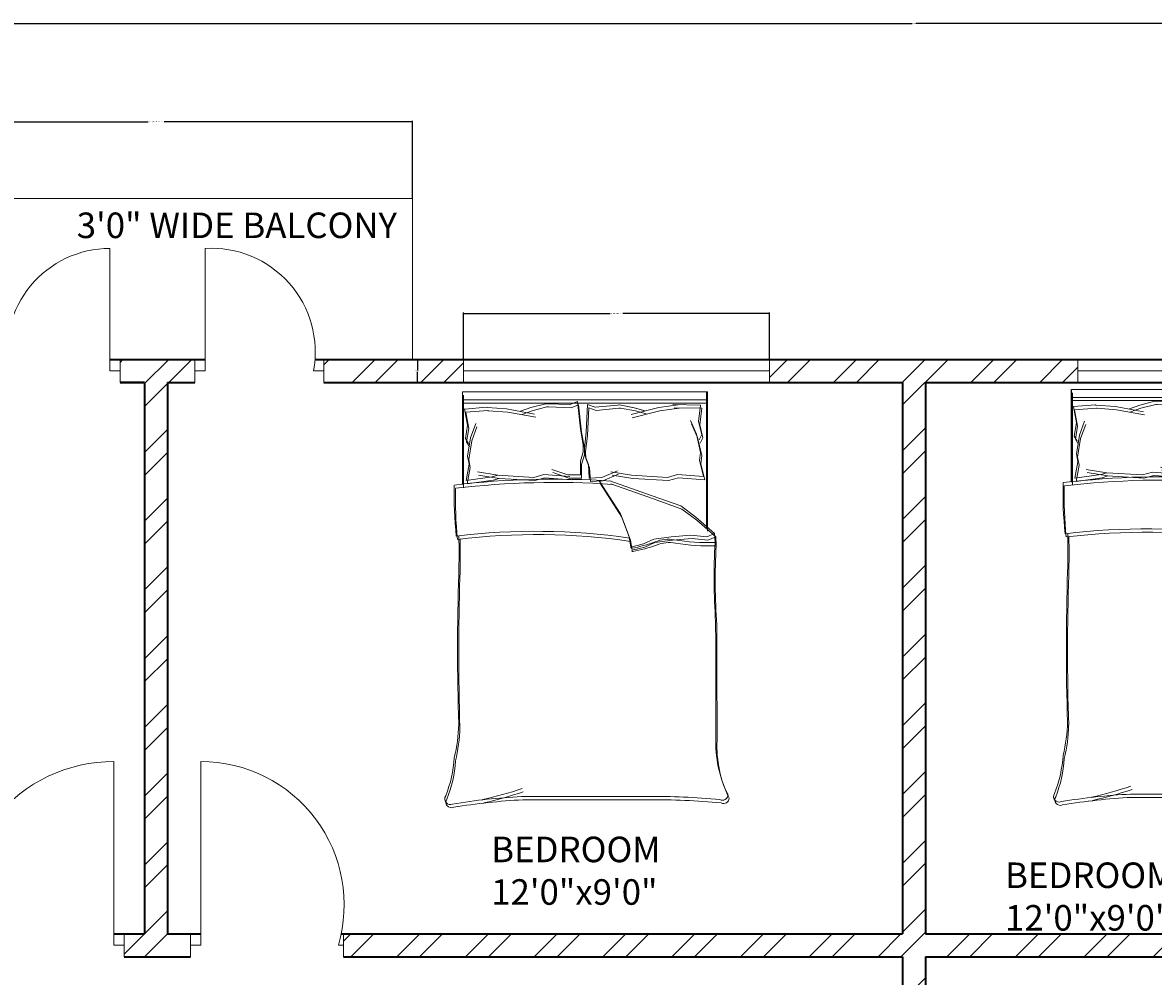
# Model space of a CAD drawing. Units: inches. Extents: x 2165 to 3042, y 1626 to 2968.
# Tile 5 of 11: x 2411 to 2633, y 2211 to 2398. Entities that reach past the tile are written whole.
import ezdxf

# ---------------------------------------------------------------- set-up
doc = ezdxf.new("R2010")
doc.units = ezdxf.units.IN
for name, color, linetype, lineweight in [('A-ANNO-DIMS', 2, 'Continuous', 18), ('A-AREA-IDEN', 7, 'Continuous', 18), ('A-DOOR', 3, 'Continuous', 18), ('A-FLOR-BALC', 7, 'Continuous', 18), ('A-FURN', 8, 'Continuous', 13), ('A-GLAZ', 4, 'Continuous', 18), ('A-WALL', 7, 'Continuous', 35), ('A-WALL-PATT', 252, 'Continuous', 13)]:
    doc.layers.add(name, color=color, linetype=linetype, lineweight=lineweight)
doc.styles.get("Standard").update_dxf_attribs({"font": 'arial.ttf'})
doc.dimstyles.get("Standard").update_dxf_attribs({"dimtxt": 0.18, "dimasz": 0.18, "dimexe": 0.18, "dimexo": 0.0625, "dimgap": 0.09, "dimtad": 0, "dimtih": 1, "dimtoh": 1, "dimdec": 4, "dimzin": 0, "dimdsep": 46, "dimtxsty": 'Standard', "dimcen": 0.09, "dimadec": 0, "dimazin": 0, "dimtfac": 1, "dimtdec": 4, "dimtofl": 0, "dimtmove": 0, "dimatfit": 3, "dimfxl": 1, "dimtolj": 1, "dimtzin": 0, "dimarcsym": 0})

# ---------------------------------------------------------------- blocks, each defined once
blk = doc.blocks.new('BED-DOUBLE')
for p, q in [((30.13, 53.18), (28.39, 53.1, 3.87)), ((30.13, 53.18), (28.39, 53.1, 3.87)), ((0, 51.27), (0, 51.49)), ((0, 51.49), (0.64, 51.49)), ((0, 51.27), (26.61, 51.27)), ((0, 51.27), (26.61, 51.27)), ((0, 51.27), (0, 3.48)), ((0.64, 51.49), (27.25, 51.49)), ((0.64, 51.49), (27.25, 51.49)), ((1.53, 3.48), (1.53, 51.27)), ((1.53, 3.47), (1.53, 51.27)), ((2.17, 3.7), (2.17, 51.49)), ((2.17, 3.7), (2.17, 51.49)), ((27.75, 52.87), (24.5, 49.16)), ((27.75, 52.87), (24.5, 49.16)), ((28.39, 53.1), (25.14, 49.39)), ((28.39, 53.1), (25.14, 49.39)), ((29.49, 52.95), (27.75, 52.87, 3.87)), ((29.49, 52.95), (27.75, 52.87, 3.87)), ((28.37, 51.33), (27.75, 52.87)), ((28.37, 51.33), (27.75, 52.87)), ((28.06, 48.23), (28.37, 51.33)), ((28.06, 48.23), (28.37, 51.33)), ((29, 51.56), (28.39, 53.1)), ((29, 51.56), (28.39, 53.1)), ((28.7, 48.46), (29, 51.56)), ((28.7, 48.46), (29, 51.56)), ((2.56, 50.11), (2.46, 44.71)), ((2.56, 50.11), (2.46, 44.71)), ((2.56, 50.11), (5.77, 49.73)), ((2.56, 50.11), (5.77, 49.73)), ((3.2, 50.34), (3.1, 44.94)), ((3.2, 50.34), (3.1, 44.94)), ((3.2, 50.34), (6.41, 49.96)), ((3.2, 50.34), (6.41, 49.96)), ((8.26, 49.31), (5.58, 48.13)), ((8.26, 49.31), (5.58, 48.13)), ((5.77, 49.73), (8.34, 50.33)), ((5.77, 49.73), (8.34, 50.33)), ((8.9, 49.54), (6.22, 48.36)), ((8.9, 49.54), (6.22, 48.36)), ((6.41, 49.96), (8.98, 50.56)), ((6.41, 49.96), (8.98, 50.56)), ((11.83, 50.11), (8.26, 49.31)), ((11.83, 50.11), (8.26, 49.31)), ((8.34, 50.33), (9.38, 49.81)), ((8.34, 50.33), (9.38, 49.81)), ((12.47, 50.34), (8.9, 49.54)), ((12.47, 50.34), (8.9, 49.54)), ((8.98, 50.56), (10.02, 50.04)), ((8.98, 50.56), (10.02, 50.04)), ((13.43, 49.92), (11.83, 50.11)), ((13.43, 49.92), (11.83, 50.11)), ((14.07, 50.15), (12.47, 50.34)), ((14.07, 50.15), (12.47, 50.34)), ((16.57, 50.7), (13.43, 49.92)), ((16.57, 50.7), (13.43, 49.92)), ((17.21, 50.93), (14.07, 50.15)), ((17.21, 50.93), (14.07, 50.15)), ((16.17, 45.57), (16.57, 50.7)), ((16.17, 45.57), (16.57, 50.7)), ((16.81, 45.79), (17.21, 50.93)), ((16.81, 45.79), (17.21, 50.93)), ((24.5, 49.16), (22.33, 46.22)), ((24.5, 49.16), (22.33, 46.22)), ((25.14, 49.39), (22.97, 46.45)), ((25.14, 49.39), (22.97, 46.45)), ((28.37, 44.36), (28.06, 48.23)), ((28.37, 44.36), (28.06, 48.23)), ((29, 44.59), (28.7, 48.46)), ((29, 44.59), (28.7, 48.46)), ((2.46, 44.71), (2.54, 45.71)), ((2.46, 44.71), (2.54, 45.71)), ((2.54, 45.71), (3.07, 41.91)), ((2.54, 45.71), (3.07, 41.91)), ((3.1, 44.94), (3.18, 45.94)), ((3.1, 44.94), (3.18, 45.94)), ((3.18, 45.94), (3.71, 42.14)), ((3.18, 45.94), (3.71, 42.14)), ((16.73, 43.61), (16.17, 45.57)), ((16.73, 43.61), (16.17, 45.57)), ((17.37, 43.83), (16.81, 45.79)), ((17.37, 43.83), (16.81, 45.79)), ((22.33, 46.22), (20.32, 40.64)), ((22.33, 46.22), (20.32, 40.64)), ((22.97, 46.45), (20.96, 40.87)), ((22.97, 46.45), (20.96, 40.87)), ((28.83, 40.95), (28.37, 44.36)), ((28.83, 40.95), (28.37, 44.36)), ((29.47, 41.18), (29, 44.59)), ((29.47, 41.18), (29, 44.59)), ((3.71, 42.14), (5.06, 36.72)), ((3.71, 42.14), (5.06, 36.72)), ((16.3, 36.6), (16.73, 43.61)), ((16.3, 36.6), (16.73, 43.61)), ((16.93, 36.82), (17.37, 43.83)), ((16.93, 36.82), (17.37, 43.83)), ((3.07, 41.91), (4.42, 36.5)), ((3.07, 41.91), (4.42, 36.49)), ((20.32, 40.64), (17.38, 32.31)), ((20.32, 40.64), (17.38, 32.31)), ((20.96, 40.87), (18.02, 32.53)), ((20.96, 40.87), (18.02, 32.53)), ((29.76, 38.94), (28.83, 40.95)), ((29.76, 38.94), (28.83, 40.95)), ((30.4, 39.17), (29.47, 41.18)), ((30.4, 39.17), (29.47, 41.18)), ((79.88, 15.29), (79.88, 39.91)), ((79.88, 15.29), (79.88, 39.91)), ((3.67, 39.2), (3.08, 37.14)), ((3.67, 39.2), (3.08, 37.13)), ((4.31, 39.43), (3.72, 37.36)), ((4.31, 39.43), (3.72, 37.36)), ((30.38, 36.46), (29.76, 38.94)), ((30.38, 36.46), (29.76, 38.94)), ((31.02, 36.69), (30.4, 39.17)), ((31.02, 36.69), (30.4, 39.17)), ((79.25, 15.06), (79.25, 39.68)), ((79.25, 15.06), (79.25, 39.68)), ((3.08, 37.14), (2.54, 34.2)), ((3.08, 37.13), (2.54, 34.2)), ((3.72, 37.36), (3.18, 34.43)), ((3.72, 37.36), (3.18, 34.43)), ((15.63, 32.56), (16.3, 36.6)), ((15.63, 32.56), (16.3, 36.6)), ((16.27, 32.79), (16.93, 36.82)), ((16.27, 32.79), (16.93, 36.82)), ((23.88, 34.45), (28.37, 36.15)), ((23.88, 34.45), (28.37, 36.15)), ((24.52, 34.68), (29, 36.38)), ((24.52, 34.68), (29, 36.38)), ((28.37, 36.15), (30.38, 36.46)), ((28.37, 36.15), (30.38, 36.46)), ((29, 36.38), (31.02, 36.69)), ((29, 36.38), (31.02, 36.69)), ((2.54, 34.2), (2.56, 33.88)), ((2.54, 34.2), (2.56, 33.88)), ((2.56, 33.88), (2.98, 29.46)), ((2.56, 33.88), (2.98, 29.46)), ((3.18, 34.43), (3.2, 34.11)), ((3.18, 34.43), (3.2, 34.11)), ((3.2, 34.11), (3.62, 29.68)), ((3.2, 34.11), (3.62, 29.68)), ((16.74, 30.75), (15.46, 33.82)), ((16.74, 30.75), (15.46, 33.82)), ((17.38, 30.98), (16.09, 34.05)), ((17.38, 30.98), (16.09, 34.05)), ((17.38, 30.26), (23.88, 34.45)), ((17.38, 30.26), (23.88, 34.45)), ((18.02, 30.49), (24.52, 34.68)), ((18.02, 30.49), (24.52, 34.68)), ((2.98, 29.46), (2.49, 27.98)), ((2.98, 29.46), (2.49, 27.98)), ((3.62, 29.68), (3.13, 28.21)), ((3.62, 29.68), (3.13, 28.21)), ((16.89, 28.3), (16.74, 30.75)), ((16.89, 28.3), (16.74, 30.75)), ((17.53, 28.53), (17.38, 30.98)), ((17.53, 28.53), (17.38, 30.98)), ((2.49, 27.98), (7.87, 27.73)), ((2.49, 27.98), (7.87, 27.73)), ((2.51, 26.21), (7.86, 26.79)), ((2.51, 26.21), (7.86, 26.79)), ((3.13, 28.21), (8.51, 27.96)), ((3.13, 28.21), (8.51, 27.96)), ((7.22, 26.56), (10.4, 27.14)), ((7.22, 26.56), (10.4, 27.14)), ((7.86, 26.79), (11.04, 27.37)), ((7.86, 26.79), (11.04, 27.37)), ((7.87, 27.73), (11.08, 27.35)), ((7.87, 27.73), (11.08, 27.35)), ((8.51, 27.96), (11.72, 27.58)), ((8.51, 27.96), (11.72, 27.58)), ((10.4, 27.14), (11.7, 27.14)), ((10.4, 27.14), (11.7, 27.14)), ((11.04, 27.37), (12.34, 27.37)), ((11.04, 27.37), (12.34, 27.37)), ((11.08, 27.35), (12.38, 27.44)), ((11.08, 27.35), (12.38, 27.44)), ((11.7, 27.14), (13.58, 26.56)), ((11.7, 27.14), (13.58, 26.56)), ((11.72, 27.58), (13.02, 27.66)), ((11.72, 27.58), (13.02, 27.66)), ((12.34, 27.37), (14.22, 26.79)), ((12.34, 27.37), (14.22, 26.79)), ((12.38, 27.44), (14.22, 28.13)), ((12.38, 27.44), (14.22, 28.13)), ((13.02, 27.66), (14.86, 28.36)), ((13.02, 27.66), (14.86, 28.36)), ((14.22, 28.13), (16.89, 28.3)), ((14.22, 28.13), (16.89, 28.3)), ((14.22, 26.79), (16.9, 26.79)), ((14.22, 26.79), (16.9, 26.79)), ((14.86, 28.36), (17.53, 28.53)), ((14.86, 28.36), (17.53, 28.53)), ((16.9, 26.79), (16.9, 24.33)), ((16.9, 26.79), (16.9, 24.33)), ((1.87, 25.98), (7.22, 26.56)), ((1.87, 25.98), (7.22, 26.56)), ((2.45, 24.54), (1.87, 25.98)), ((2.45, 24.54), (1.87, 25.98)), ((2.3, 20.09), (2.45, 24.54)), ((2.3, 20.09), (2.45, 24.54)), ((3.09, 24.77), (2.51, 26.21)), ((3.09, 24.77), (2.51, 26.21)), ((2.94, 20.32), (3.09, 24.77)), ((2.94, 20.32), (3.09, 24.77)), ((13.58, 26.56), (16.26, 26.56)), ((13.58, 26.56), (16.26, 26.56)), ((16.17, 19.38), (16.57, 24.52)), ((16.17, 19.38), (16.57, 24.52)), ((16.26, 26.56), (16.26, 24.1)), ((16.26, 26.56), (16.26, 24.1)), ((16.81, 19.61), (17.21, 24.74)), ((16.81, 19.61), (17.21, 24.74)), ((16.26, 24.1), (15.17, 20.96)), ((16.26, 24.1), (15.17, 20.96)), ((16.9, 24.33), (15.81, 21.19)), ((16.9, 24.33), (15.81, 21.19)), ((2.3, 19.77), (2.3, 20.09)), ((2.3, 19.77), (2.3, 20.09)), ((2.94, 20), (2.94, 20.32)), ((2.94, 20), (2.94, 20.32)), ((3.67, 17.11), (2.94, 20)), ((3.67, 17.11), (2.94, 20)), ((3.03, 16.88), (2.3, 19.77)), ((3.03, 16.88), (2.3, 19.77)), ((3.96, 12.34), (4.97, 17.83)), ((3.96, 12.34), (4.97, 17.83)), ((16.73, 17.42), (16.17, 19.38)), ((16.73, 17.42), (16.17, 19.38)), ((17.37, 17.65), (16.81, 19.61)), ((17.37, 17.65), (16.81, 19.61)), ((3.75, 14.85), (3.03, 16.88)), ((3.75, 14.85), (3.03, 16.88)), ((3.32, 12.11), (4.33, 17.6)), ((3.32, 12.11), (4.33, 17.6)), ((4.39, 15.08), (3.67, 17.11)), ((4.39, 15.08), (3.67, 17.11)), ((16.3, 10.41), (16.73, 17.42)), ((16.3, 10.41), (16.73, 17.42)), ((16.93, 10.64), (17.37, 17.65)), ((16.93, 10.64), (17.37, 17.65)), ((3.03, 8.28), (3.32, 12.11)), ((3.03, 8.28), (3.32, 12.11)), ((3.67, 8.51), (3.96, 12.34)), ((3.67, 8.51), (3.96, 12.34)), ((15.63, 6.38), (16.3, 10.41)), ((15.63, 6.38), (16.3, 10.41)), ((16.27, 6.61), (16.93, 10.64)), ((16.27, 6.61), (16.93, 10.64)), ((16.3, 10.41), (16.62, 9.28)), ((16.3, 10.41), (16.62, 9.28)), ((16.62, 9.28), (17.34, 4.18)), ((16.62, 9.28), (17.34, 4.18)), ((16.93, 10.64), (17.26, 9.51)), ((16.93, 10.64), (17.26, 9.51)), ((17.26, 9.51), (17.98, 4.41)), ((17.26, 9.51), (17.98, 4.41)), ((3.01, 8.18), (3.03, 8.28)), ((3.01, 8.18), (3.03, 8.28)), ((3.34, 3.9), (3.01, 8.18)), ((3.34, 3.9), (3.01, 8.18)), ((3.65, 8.41), (3.67, 8.51)), ((3.65, 8.41), (3.67, 8.51)), ((3.98, 4.13), (3.65, 8.41)), ((3.98, 4.13), (3.65, 8.41)), ((3.32, 3.89), (6.5, 4.47)), ((3.32, 3.89), (6.5, 4.47)), ((3.96, 4.12), (7.14, 4.7)), ((3.96, 4.12), (7.14, 4.7)), ((8.96, 5.05), (6.21, 6.06)), ((8.96, 5.05), (6.21, 6.06)), ((6.5, 4.47), (9.1, 4.04)), ((6.5, 4.47), (9.1, 4.04)), ((9.59, 5.28), (6.85, 6.29)), ((9.59, 5.28), (6.85, 6.29)), ((7.14, 4.7), (9.74, 4.27)), ((7.14, 4.7), (9.74, 4.27)), ((12.57, 4.47), (8.96, 5.05)), ((12.57, 4.47), (8.96, 5.05)), ((9.1, 4.04), (10.11, 4.62)), ((9.1, 4.04), (10.11, 4.62)), ((13.21, 4.7), (9.59, 5.28)), ((13.21, 4.7), (9.59, 5.28)), ((9.74, 4.27), (10.75, 4.85)), ((9.74, 4.27), (10.75, 4.85)), ((14.16, 4.76), (12.57, 4.47)), ((14.16, 4.76), (12.57, 4.47)), ((14.8, 4.99), (13.21, 4.7)), ((14.8, 4.99), (13.21, 4.7)), ((17.34, 4.18), (14.16, 4.76)), ((17.34, 4.18), (14.16, 4.76)), ((17.98, 4.41), (14.8, 4.99)), ((17.98, 4.41), (14.8, 4.99)), ((18.11, 3.48), (0, 3.48)), ((18.11, 3.47), (0, 3.47)), ((18.75, 3.7), (0.64, 3.7)), ((18.75, 3.7), (0.64, 3.7))]:
    blk.add_line(p, q)
for centre, radius, start, end in [((68.67, 76.16), 23.07, 267.4714, 296.4681), ((68.67, 76.16), 23.07, 267.4714, 296.4681), ((69.31, 76.39), 23.07, 267.4714, 296.4681), ((69.31, 76.39), 23.07, 267.4714, 296.4681), ((78.87, 54.41), 1.1, 332.6588, 86.02), ((78.87, 54.41), 1.1, 332.6588, 86.02), ((79.51, 54.64), 1.1, 332.6588, 86.02), ((79.51, 54.64), 1.1, 332.6588, 86.02), ((-6.02, 51.56), 36.18, 349.8763, 2.5657), ((-6.02, 51.56), 36.18, 349.8763, 2.5657), ((36.95, 182.49), 129.5, 266.9791, 273.8365), ((36.95, 182.49), 129.5, 266.9791, 273.8365), ((68.46, -4508.52), 4561.86, 90.00217, 90.28689), ((68.46, -4508.52), 4561.86, 90.00217, 90.28689), ((212.28, 41.15), 133.04, 174.4998, 180.6351), ((212.28, 41.15), 133.04, 174.4998, 180.6351), ((212.92, 41.38), 133.04, 174.4998, 180.6351), ((212.92, 41.38), 133.04, 174.4998, 180.6351), ((-6.66, 51.33), 36.18, 349.8763, 2.5657), ((-6.66, 51.33), 36.18, 349.8763, 2.5657), ((36.32, 182.27), 129.5, 266.9791, 273.8365), ((36.32, 182.27), 129.5, 266.9791, 273.8365), ((67.82, -4508.74), 4561.86, 90.00217, 90.28689), ((67.82, -4508.74), 4561.86, 90.00217, 90.28689), ((35.07, 43.74), 6.22, 168.6608, 203.7384), ((35.07, 43.74), 6.22, 168.6608, 203.7384), ((35.71, 43.97), 6.22, 168.6608, 203.7384), ((35.71, 43.97), 6.22, 168.6608, 203.7384), ((1.48, 31.15), 29.65, 10.6617, 19.8806), ((1.48, 31.15), 29.65, 10.6617, 19.8806), ((2.12, 31.38), 29.65, 10.6617, 19.8806), ((2.12, 31.38), 29.65, 10.6617, 19.8806), ((156.32, 17.76), 129.02, 171.7845, 186.9006), ((156.32, 17.76), 129.02, 171.7845, 186.9006), ((156.96, 17.98), 129.02, 171.7845, 186.9006), ((156.96, 17.98), 129.02, 171.7845, 186.9006), ((30.44, 36.64), 0.185, 250.2464, 1.1377), ((30.44, 36.64), 0.185, 250.2464, 1.1377), ((31.08, 36.86), 0.185, 250.2464, 1.1377), ((31.08, 36.86), 0.185, 250.2464, 1.1377), ((182.05, 21.36), 164.97, 176.0865, 186.7821), ((182.05, 21.36), 164.97, 176.0865, 186.7821), ((182.69, 21.59), 164.97, 176.0865, 186.7821), ((182.69, 21.59), 164.97, 176.0865, 186.7821), ((-23.71, -17.22), 106.46, 13.3832, 17.7053), ((-23.71, -17.22), 106.46, 13.3832, 17.7053), ((-23.07, -16.99), 106.46, 13.3832, 17.7053), ((-23.07, -16.99), 106.46, 13.3832, 17.7053), ((200.84, 21.43), 121.76, 182.9958, 189.4091), ((200.84, 21.43), 121.76, 182.9958, 189.4091), ((201.48, 21.66), 121.76, 182.9958, 189.4091), ((201.48, 21.65), 121.76, 182.9958, 189.4091), ((20.1, 85.16), 83.31, 268.7218, 275.604), ((20.1, 85.16), 83.31, 268.7218, 275.604), ((20.74, 85.39), 83.31, 268.7218, 275.604), ((20.74, 85.39), 83.31, 268.7218, 275.604), ((31.17, -167.31), 170.11, 88.4762, 91.0082), ((31.17, -167.31), 170.11, 88.4762, 91.0082), ((31.81, -167.08), 170.11, 88.4762, 91.0082), ((31.81, -167.08), 170.11, 88.4762, 91.0082), ((50.61, 484.82), 482.31, 268.2277, 271.7185), ((50.61, 484.82), 482.31, 268.2277, 271.7185), ((51.25, 485.05), 482.31, 268.2277, 271.7185), ((51.25, 485.05), 482.31, 268.2277, 271.7185), ((64.52, -26.9), 29.63, 76.0648, 88.9113), ((64.52, -26.9), 29.63, 76.0648, 88.9113), ((65.15, -26.67), 29.63, 76.0648, 88.9113), ((65.15, -26.67), 29.63, 76.0648, 88.9113), ((70.28, -21.66), 23.56, 67.9751, 86.652), ((70.28, -21.66), 23.56, 67.9751, 86.652), ((70.92, -21.43), 23.56, 67.9751, 86.652), ((70.92, -21.43), 23.56, 67.9751, 86.652), ((79.72, 1.09), 1.09, 236.1736, 23.4781), ((79.72, 1.09), 1.09, 236.1736, 23.4781), ((80.36, 1.32), 1.09, 236.1736, 23.4781), ((80.36, 1.32), 1.09, 236.1736, 23.4781)]:
    blk.add_arc(centre, radius, start, end)
blk = doc.blocks.new('BALCONY-RAIL-PLAN')
for p, q in [((0, 31.5), (0, 0)), ((100.5, 31.5), (100.5, 0)), ((100.5, 0), (0, 0))]:
    blk.add_line(p, q)
blk = doc.blocks.new('WIN-60-B')
for p, q in [((0, 4.5), (0, 0)), ((60, 2.25), (60, 4.5)), ((60, 4.5), (60, 0)), ((0, 0), (0, 2.25)), ((0, 2.25), (60, 2.25))]:
    blk.add_line(p, q)
blk = doc.blocks.new('*D24')
at = {"layer": 'A-ANNO-DIMS', "color": 0, "lineweight": -2, "transparency": 16777216}
for p, q in [((2387.1, 2363.64), (2387.1, 2378.83)), ((2387.28, 2378.65), (2435.81, 2378.65)), ((2487.42, 2378.65), (2438.9, 2378.65)), ((2487.6, 2363.64), (2487.6, 2378.83))]:
    blk.add_line(p, q, dxfattribs=at)
at = {"layer": 'A-ANNO-DIMS', "color": 0, "transparency": 16777216}
for points in [[(2387.28, 2378.68), (2387.28, 2378.62), (2387.1, 2378.65)], [(2487.42, 2378.68), (2487.42, 2378.62), (2487.6, 2378.65)]]:
    blk.add_solid(points, dxfattribs=at)
at = {"layer": 'Defpoints', "color": 0, "transparency": 16777216}
for p in [(2387.1, 2378.65), (2387.1, 2363.58), (2487.6, 2363.58)]:
    blk.add_point(p, dxfattribs=at)
at = {"layer": 'A-ANNO-DIMS', "color": 0, "transparency": 16777216, "insert": (2437.35, 2378.65), "char_height": 0.18, "attachment_point": 5}
blk.add_mtext('\\A1;BALCONY RAIL 101 TYP.', dxfattribs=at)
blk = doc.blocks.new('*D26')
at = {"layer": 'A-ANNO-DIMS', "color": 0, "lineweight": -2, "transparency": 16777216}
for p, q in [((2497.54, 2332.14), (2497.54, 2341.26)), ((2497.72, 2341.08), (2526.3, 2341.08)), ((2557.36, 2341.08), (2528.78, 2341.08)), ((2557.54, 2332.14), (2557.54, 2341.26))]:
    blk.add_line(p, q, dxfattribs=at)
at = {"layer": 'A-ANNO-DIMS', "color": 0, "transparency": 16777216}
for points in [[(2497.72, 2341.11), (2497.72, 2341.05), (2497.54, 2341.08)], [(2557.36, 2341.11), (2557.36, 2341.05), (2557.54, 2341.08)]]:
    blk.add_solid(points, dxfattribs=at)
at = {"layer": 'Defpoints', "color": 0, "transparency": 16777216}
for p in [(2557.54, 2341.08), (2497.54, 2332.08), (2557.54, 2332.08)]:
    blk.add_point(p, dxfattribs=at)
at = {"layer": 'A-ANNO-DIMS', "color": 0, "transparency": 16777216, "insert": (2527.54, 2341.08), "char_height": 0.18, "attachment_point": 5}
blk.add_mtext('\\A1;WINDOW B 60 TYP.', dxfattribs=at)
blk = doc.blocks.new('*D27')
at = {"layer": 'A-ANNO-DIMS', "color": 0, "lineweight": -2, "transparency": 16777216}
for p, q in [((2497.48, 2332.08), (2488.36, 2332.08)), ((2488.54, 2331.9), (2488.54, 2330.01)), ((2488.54, 2327.76), (2488.54, 2329.65)), ((2497.48, 2327.58), (2488.36, 2327.58))]:
    blk.add_line(p, q, dxfattribs=at)
at = {"layer": 'A-ANNO-DIMS', "color": 0, "transparency": 16777216}
for points in [[(2488.51, 2331.9), (2488.57, 2331.9), (2488.54, 2332.08)], [(2488.51, 2327.76), (2488.57, 2327.76), (2488.54, 2327.58)]]:
    blk.add_solid(points, dxfattribs=at)
at = {"layer": 'Defpoints', "color": 0, "transparency": 16777216}
for p in [(2488.54, 2332.08), (2497.54, 2332.08), (2497.54, 2327.58)]:
    blk.add_point(p, dxfattribs=at)
at = {"layer": 'A-ANNO-DIMS', "color": 0, "transparency": 16777216, "insert": (2488.54, 2329.83), "char_height": 0.18, "attachment_point": 5}
blk.add_mtext('\\A1;5 TYP.', dxfattribs=at)
blk = doc.blocks.new('*D50')
at = {"layer": 'A-ANNO-DIMS', "color": 0, "lineweight": -2, "transparency": 16777216}
for p, q in [((2286.6, 2332.14), (2286.6, 2398.06)), ((2286.78, 2397.88), (2585.46, 2397.88)), ((2884.92, 2397.88), (2586.25, 2397.88)), ((2885.1, 2332.14), (2885.1, 2398.06))]:
    blk.add_line(p, q, dxfattribs=at)
at = {"layer": 'A-ANNO-DIMS', "color": 0, "transparency": 16777216}
for points in [[(2286.78, 2397.91), (2286.78, 2397.85), (2286.6, 2397.88)], [(2884.92, 2397.91), (2884.92, 2397.85), (2885.1, 2397.88)]]:
    blk.add_solid(points, dxfattribs=at)
at = {"layer": 'Defpoints', "color": 0, "transparency": 16777216}
for p in [(2885.1, 2397.88), (2286.6, 2332.08), (2885.1, 2332.08)]:
    blk.add_point(p, dxfattribs=at)
at = {"layer": 'A-ANNO-DIMS', "color": 0, "transparency": 16777216, "insert": (2585.85, 2397.88), "char_height": 0.18, "attachment_point": 5}
blk.add_mtext('\\A1;598.5', dxfattribs=at)
blk = doc.blocks.new('*D51')
at = {"layer": 'A-ANNO-DIMS', "color": 0, "lineweight": -2, "transparency": 16777216}
for p, q in [((2387.04, 2363.58), (2252.12, 2363.58)), ((2252.3, 2363.4), (2252.3, 2082.76)), ((2252.3, 1801.76), (2252.3, 2082.4)), ((2535.54, 1801.58), (2252.12, 1801.58))]:
    blk.add_line(p, q, dxfattribs=at)
at = {"layer": 'A-ANNO-DIMS', "color": 0, "transparency": 16777216}
for points in [[(2252.27, 2363.4), (2252.33, 2363.4), (2252.3, 2363.58)], [(2252.27, 1801.76), (2252.33, 1801.76), (2252.3, 1801.58)]]:
    blk.add_solid(points, dxfattribs=at)
at = {"layer": 'Defpoints', "color": 0, "transparency": 16777216}
for p in [(2252.3, 2363.58), (2387.1, 2363.58), (2535.6, 1801.58)]:
    blk.add_point(p, dxfattribs=at)
at = {"layer": 'A-ANNO-DIMS', "color": 0, "transparency": 16777216, "insert": (2252.3, 2082.58), "char_height": 0.18, "attachment_point": 5}
blk.add_mtext('\\A1;562', dxfattribs=at)

msp = doc.modelspace()

# ---------------------------------------------------------------- hatches: boundary and pattern name
at = {"layer": 'A-WALL-PATT'}
h = msp.add_hatch(dxfattribs=at)
h.set_pattern_fill('ANSI32', color=256)
h.paths.add_polyline_path([(2406.4931, 2332.0783), (2286.6045, 2332.0783), (2286.6045, 2310.967), (2288.8545, 2310.967), (2291.1045, 2310.967), (2291.1045, 2327.5783), (2406.4931, 2327.5783), (2406.4931, 2329.8283)])
h.paths.add_polyline_path([(2439.6045, 2327.5783), (2444.9584, 2327.5783), (2444.9584, 2332.0783), (2430.2901, 2332.0783), (2430.2901, 2329.8283), (2430.2901, 2327.5783), (2435.1045, 2327.5783), (2435.1045, 2219.5783), (2431.0902, 2219.5783), (2431.0902, 2215.0783), (2435.1045, 2215.0783), (2444.1108, 2215.0783), (2444.1108, 2217.3283), (2444.1108, 2219.5783), (2439.6045, 2219.5783)])
h.paths.add_polyline_path([(2497.5418, 2329.8283), (2497.5418, 2332.0783), (2470.1978, 2332.0783), (2470.1978, 2327.5783), (2497.5418, 2327.5783)])
h.paths.add_polyline_path([(2617.9543, 2332.0783), (2557.5418, 2332.0783), (2557.5418, 2327.5783), (2583.6045, 2327.5783), (2583.6045, 2219.5783), (2474.0523, 2219.5783), (2474.0523, 2215.0783), (2583.6045, 2215.0783), (2583.6045, 2107.0783), (2579.3609, 2107.0783), (2579.3609, 2102.5783), (2588.1045, 2102.5783), (2593.5283, 2102.5783), (2593.5283, 2104.8283), (2593.5283, 2107.0783), (2588.1045, 2107.0783), (2588.1045, 2215.0783), (2691.2325, 2215.0783), (2691.2325, 2217.3283), (2691.2325, 2219.5783), (2588.1045, 2219.5783), (2588.1045, 2327.5783), (2617.9543, 2327.5783)])
h.paths.add_polyline_path([(2702.4444, 2329.8283), (2702.4444, 2332.0783), (2677.9543, 2332.0783), (2677.9543, 2327.5783), (2702.4444, 2327.5783)])
h.paths.add_polyline_path([(2736.6045, 2327.5783), (2742.5161, 2327.5783), (2742.5161, 2329.8283), (2742.5161, 2332.0783), (2727.7639, 2332.0783), (2727.7639, 2329.8283), (2727.7639, 2327.5783), (2732.1045, 2327.5783), (2732.1045, 2219.5783), (2726.4404, 2219.5783), (2726.4404, 2215.0783), (2732.1045, 2215.0783), (2742.7291, 2215.0783), (2742.7291, 2217.3283), (2742.7291, 2219.5783), (2736.6045, 2219.5783)])
h.paths.add_polyline_path([(2885.1045, 2332.0783), (2768.4887, 2332.0783), (2768.4887, 2327.5783), (2784.6045, 2327.5783), (2880.6045, 2327.5783), (2880.6045, 2310.967), (2885.1045, 2310.967)])
h.paths.add_polyline_path([(2885.1045, 2250.967), (2880.6045, 2250.967), (2880.6045, 2219.5783), (2776.5755, 2219.5783), (2776.5755, 2215.0783), (2788.1045, 2215.0783), (2788.1045, 2209.8634), (2790.3545, 2209.8634), (2792.6045, 2209.8634), (2792.6045, 2215.0783), (2880.6045, 2215.0783), (2880.6045, 2139.0783), (2871.2037, 2139.0783), (2871.2037, 2134.5783), (2885.1045, 2134.5783)])
h.paths.add_polyline_path([(2545.013, 2107.0783), (2474.0523, 2107.0783), (2291.1045, 2107.0783), (2291.1045, 2102.5783), (2535.6045, 2102.5783), (2535.6045, 2096.8046), (2537.8545, 2096.8046), (2540.1045, 2096.8046), (2540.1045, 2102.5783), (2545.013, 2102.5783), (2545.013, 2104.8283)])
h.paths.add_polyline_path([(2397.7297, 2217.3283), (2397.7297, 2219.5783), (2291.1045, 2219.5783), (2291.1045, 2250.967), (2286.6045, 2250.967), (2286.6045, 2206.1346), (2288.8545, 2206.1346), (2291.1045, 2206.1346), (2291.1045, 2215.0783), (2367.1045, 2215.0783), (2367.1045, 2212.2868), (2371.6045, 2212.2868), (2371.6045, 2215.0783), (2397.7297, 2215.0783)])
h.paths.add_polyline_path([(2291.1045, 1978.5783), (2367.1045, 1978.5783), (2371.6045, 1978.5783), (2373.2641, 1978.5783), (2374.4883, 1978.5783), (2374.4883, 1980.8283), (2374.4883, 1983.0783), (2371.6045, 1983.0783), (2371.6045, 1986.964), (2369.9051, 1986.964), (2369.3545, 1986.964), (2367.1045, 1986.964), (2367.1045, 1983.0783), (2291.1045, 1983.0783), (2291.1045, 2001.1808), (2286.6045, 2001.1808), (2286.6045, 1947.0203), (2288.8545, 1947.0203), (2291.1045, 1947.0203)])
h.paths.add_polyline_path([(2291.1045, 1887.0203), (2286.6045, 1887.0203), (2286.6045, 1842.0783), (2381.2561, 1842.0783), (2381.2561, 1844.3283), (2381.2561, 1846.5783), (2363.1045, 1846.5783), (2291.1045, 1846.5783)])
h.paths.add_polyline_path([(2415.6045, 1978.5783), (2421.1681, 1978.5783), (2421.1681, 1983.0783), (2415.6045, 1983.0783), (2406.5227, 1983.0783), (2406.5227, 1980.8283), (2406.5227, 1978.5783), (2411.1045, 1978.5783), (2411.1045, 1846.5783), (2406.7549, 1846.5783), (2406.7549, 1842.0783), (2419.2885, 1842.0783), (2419.2885, 1844.3283), (2419.2885, 1846.5783), (2415.6045, 1846.5783)])
h.paths.add_polyline_path([(2586.6045, 1982.779), (2586.6045, 1991.5911), (2582.1045, 1991.5911), (2582.1045, 1982.779), (2540.1045, 1982.779), (2540.1045, 2036.779), (2582.1045, 2036.779), (2582.1045, 2027.6051), (2586.6045, 2027.6051), (2586.6045, 2041.279), (2582.1045, 2041.279), (2540.1045, 2041.279), (2540.1045, 2063.9064), (2537.8545, 2063.9064), (2535.6045, 2063.9064), (2535.6045, 1983.0783), (2455.068, 1983.0783), (2455.068, 1978.5783), (2535.6045, 1978.5783), (2535.6045, 1846.5783), (2522.622, 1846.5783), (2522.622, 1842.0783), (2535.6045, 1842.0783), (2535.6045, 1806.0783), (2535.6045, 1801.5783), (2556.726, 1801.5783), (2556.726, 1803.8283), (2556.726, 1806.0783), (2540.1045, 1806.0783), (2540.1045, 1842.0783), (2540.1045, 1846.5783), (2540.1045, 1978.279), (2586.6045, 1978.279)])
h.paths.add_polyline_path([(2636.1045, 1978.5783), (2717.6642, 1978.5783), (2717.6642, 1980.8283), (2717.6642, 1983.0783), (2636.1045, 1983.0783), (2636.1045, 2063.9064), (2633.8545, 2063.9064), (2631.6045, 2063.9064), (2631.6045, 1846.5783), (2631.6045, 1842.0783), (2631.6045, 1806.0783), (2604.726, 1806.0783), (2604.726, 1801.5783), (2636.1045, 1801.5783), (2636.1045, 1842.0783), (2644.3411, 1842.0783), (2644.3411, 1844.3283), (2644.3411, 1846.5783), (2636.1045, 1846.5783)])
h.paths.add_polyline_path([(2760.6045, 1978.5783), (2764.9931, 1978.5783), (2764.9931, 1983.0783), (2750.4727, 1983.0783), (2750.4727, 1980.8283), (2750.4727, 1978.5783), (2756.1045, 1978.5783), (2756.1045, 1846.5783), (2749.4543, 1846.5783), (2749.4543, 1842.0783), (2765.1894, 1842.0783), (2765.1894, 1846.5783), (2760.6045, 1846.5783)])
h.paths.add_polyline_path([(2880.6045, 1983.0783), (2804.6045, 1983.0783), (2804.6045, 1988.3825), (2802.3545, 1988.3825), (2800.1045, 1988.3825), (2800.1045, 1983.0783), (2800.1045, 1978.5783), (2880.6045, 1978.5783)])
h.paths.add_polyline_path([(2885.1045, 2075.5783), (2871.2037, 2075.5783), (2871.2037, 2071.0783), (2880.6045, 2071.0783), (2880.6045, 1948.8144), (2885.1045, 1948.8144)])
h.paths.add_polyline_path([(2885.1045, 1888.8144), (2880.6045, 1888.8144), (2880.6045, 1846.5783), (2792.1167, 1846.5783), (2792.1167, 1842.0783), (2885.1045, 1842.0783)])
h.paths.add_polyline_path([(2724.4848, 1846.5783), (2708.1045, 1846.5783), (2692.3411, 1846.5783), (2692.3411, 1842.0783), (2724.4848, 1842.0783), (2724.4848, 1844.3283)])
h.paths.add_polyline_path([(2474.622, 1844.4672), (2474.622, 1846.5783), (2444.7417, 1846.5783), (2444.7417, 1842.0783), (2474.622, 1842.0783)])

# ---------------------------------------------------------------- linework, layer by layer
at = {"layer": 'A-DOOR'}
for p, q in [((2428.2901, 2329.8283), (2428.2901, 2353.8283)), ((2446.9584, 2329.8283), (2446.9584, 2353.8283)), ((2430.2901, 2327.5783), (2430.2901, 2332.0783)), ((2430.2901, 2332.0783), (2430.2901, 2329.8283)), ((2444.9584, 2327.5783), (2444.9584, 2332.0783)), ((2444.9584, 2332.0783), (2444.9584, 2329.8283)), ((2470.1978, 2332.0783), (2470.1978, 2327.5783)), ((2430.2901, 2329.8283), (2428.2901, 2329.8283)), ((2444.9584, 2329.8283), (2446.9584, 2329.8283)), ((2470.1978, 2329.8283), (2468.1978, 2329.8283)), ((2470.1978, 2327.5783), (2470.1978, 2329.8283)), ((2429.0902, 2217.3283), (2429.0902, 2253.3283)), ((2446.1108, 2217.3283), (2446.1108, 2253.3283)), ((2431.0902, 2219.5783), (2431.0902, 2215.0783)), ((2444.1108, 2219.5783), (2444.1108, 2215.0783)), ((2474.0523, 2219.5783), (2474.0523, 2215.0783)), ((2431.0902, 2217.3283), (2429.0902, 2217.3283)), ((2431.0902, 2215.0783), (2431.0902, 2217.3283)), ((2444.1108, 2215.0783), (2444.1108, 2217.3283)), ((2444.1108, 2217.3283), (2446.1108, 2217.3283)), ((2474.0523, 2217.3283), (2473.0523, 2217.3283)), ((2474.0523, 2215.0783), (2474.0523, 2217.3283))]:
    msp.add_line(p, q, dxfattribs=at)
for centre, radius, start, end in [((2428.2901, 2333.6633), 20.165, 90, 190.963229), ((2448.1841, 2333.5149), 20.3504, 349.562896, 93.452968), ((2429.0902, 2223.3556), 29.9727, 90, 191.600845), ((2446.1108, 2225.2471), 28.0812, 343.620502, 90)]:
    msp.add_arc(centre, radius, start, end, dxfattribs=at)
at = {"layer": 'A-WALL'}
for p, q in [((2428.2901, 2332.0783), (2446.9584, 2332.0783)), ((2428.2901, 2332.0783), (2446.9584, 2332.0783)), ((2468.4837, 2332.0783), (2704.2966, 2332.0783)), ((2468.4837, 2332.0783), (2704.2966, 2332.0783)), ((2435.1045, 2327.5783), (2430.2901, 2327.5783)), ((2430.2901, 2327.5783), (2435.1045, 2327.5783)), ((2435.1045, 2327.5783), (2435.1045, 2219.5783)), ((2439.6045, 2327.5783), (2439.6045, 2219.5783)), ((2439.6045, 2327.5783), (2444.9584, 2327.5783)), ((2439.6045, 2327.5783), (2444.9584, 2327.5783)), ((2470.1978, 2327.5783), (2487.6045, 2327.5783)), ((2470.1978, 2327.5783), (2583.6045, 2327.5783)), ((2583.6045, 2327.5783), (2583.6045, 2219.5783)), ((2588.1045, 2327.5783), (2588.1045, 2219.5783)), ((2588.1045, 2327.5783), (2702.4444, 2327.5783)), ((2429.0902, 2219.5783), (2435.1045, 2219.5783)), ((2439.6045, 2219.5783), (2446.1108, 2219.5783)), ((2473.6138, 2219.5783), (2583.6045, 2219.5783)), ((2588.1045, 2219.5783), (2692.992, 2219.5783)), ((2431.0902, 2215.0783), (2435.1045, 2215.0783)), ((2435.1045, 2215.0783), (2444.1108, 2215.0783)), ((2474.0523, 2215.0783), (2583.6045, 2215.0783)), ((2583.6045, 2215.0783), (2583.6045, 2107.0783)), ((2588.1045, 2215.0783), (2691.2325, 2215.0783)), ((2588.1045, 2215.0783), (2588.1045, 2107.0783))]:
    msp.add_line(p, q, dxfattribs=at)

# ---------------------------------------------------------------- block references
at = {"layer": 'A-FLOR-BALC', "rotation": 180}
msp.add_blockref('BALCONY-RAIL-PLAN', (2487.6049, 2363.5786), dxfattribs=at)
at = {"layer": 'A-FURN'}
for p, rotation in [((2613.1768, 2326.1825), 269.9999998332427), ((2493.9016, 2325.7149), 269.9999998332426)]:
    msp.add_blockref('BED-DOUBLE', p, dxfattribs=dict(at, rotation=rotation))
at = {"layer": 'A-GLAZ'}
msp.add_blockref('WIN-60-B', (2497.542, 2327.578), dxfattribs=at)
at = {"layer": 'A-GLAZ', "extrusion": (0, 0, -1), "zscale": -1, "rotation": 180}
msp.add_blockref('WIN-60-B', (-2617.9544, 2332.0786), dxfattribs=at)

# ---------------------------------------------------------------- texts
at = {"layer": 'A-AREA-IDEN', "char_height": 5, "attachment_point": 1}
for s, width, insert in [('3\'0" WIDE BALCONY', 69.420923, (2421.7957, 2360.8547)), ('BEDROOM\\P12\'0"x9\'0"', 104.85241, (2502.9978, 2238.601)), ('BEDROOM\\P12\'0"x9\'0"', 99.842091, (2603.6657, 2233.5451))]:
    msp.add_mtext_dynamic_manual_height_columns(s, width=width, gutter_width=12.5, heights=[0], dxfattribs=dict(at, insert=insert))

# ---------------------------------------------------------------- dimensions: what is measured, and where the dimension line sits
at = {"layer": 'A-ANNO-DIMS'}
dim = msp.add_linear_dim(base=(2885.1045, 2397.8783), p1=(2286.6045, 2332.0783), p2=(2885.1045, 2332.0783), dimstyle='Standard', override={"dimdec": 1, "dimlfac": 1, "dimrnd": 0, "dimzin": 0, "dimdsep": 46, "dimlunit": 2}, dxfattribs=at)
dim.commit()
dim.dimension.update_dxf_attribs({"geometry": '*D50', "text_midpoint": (2585.8545, 2397.8783)})
for base, p1, p2, angle, text, picture, middle in [((2387.1044518572, 2378.6533076613), (2487.6044518572, 2363.5783076613), (2387.1044518572, 2363.5783076613), 180, 'BALCONY RAIL <> TYP.', '*D24', (2437.3544518572, 2378.6533076613)), ((2488.541827055, 2332.0783076613), (2497.541827055, 2327.5783076613), (2497.541827055, 2332.0783076613), 90, '<> TYP.', '*D27', (2488.541827055, 2329.8283076613))]:
    dim = msp.add_linear_dim(base=base, p1=p1, p2=p2, angle=angle, text=text, dimstyle='Standard', override={"dimdec": 0, "dimlfac": 1, "dimrnd": 0, "dimzin": 0, "dimdsep": 46, "dimlunit": 2}, dxfattribs=at)
    dim.commit()
    dim.dimension.update_dxf_attribs({"geometry": picture, "text_midpoint": middle})
dim = msp.add_linear_dim(base=(2252.3045, 2363.5783), p1=(2535.6045, 1801.5783), p2=(2387.1045, 2363.5783), angle=90, dimstyle='Standard', override={"dimdec": 0, "dimlfac": 1, "dimrnd": 0, "dimzin": 0, "dimdsep": 46, "dimlunit": 2}, dxfattribs=at)
dim.commit()
dim.dimension.update_dxf_attribs({"geometry": '*D51', "text_midpoint": (2252.3045, 2082.5783)})
dim = msp.add_linear_dim(base=(2557.5418, 2341.0783), p1=(2497.5418, 2332.0783), p2=(2557.5418, 2332.0783), text='WINDOW B <> TYP.', dimstyle='Standard', override={"dimdec": 0, "dimlfac": 1, "dimrnd": 0, "dimzin": 0, "dimdsep": 46, "dimlunit": 2}, dxfattribs=at)
dim.commit()
dim.dimension.update_dxf_attribs({"geometry": '*D26', "text_midpoint": (2527.5418, 2341.0783)})

doc.saveas('drawing.dxf')
